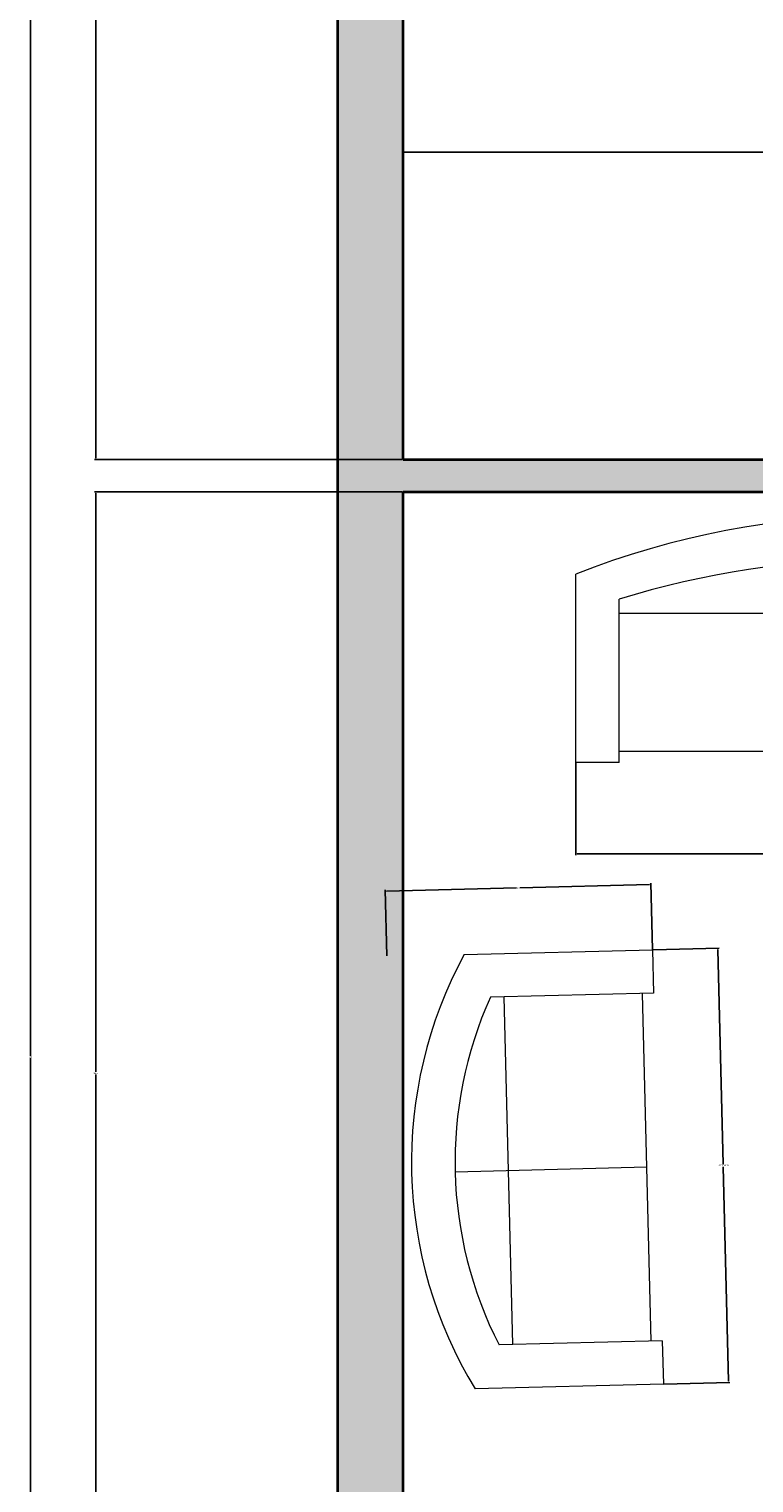
# Model space of a CAD drawing. Units: inches. Extents: x 1563 to 2428, y 777 to 1464.
# Tile 3 of 11: x 1563 to 1663, y 1063 to 1263. Entities that reach past the tile are written whole.
import ezdxf

# ---------------------------------------------------------------- set-up
doc = ezdxf.new("R2010")
doc.units = ezdxf.units.IN
for name, color, linetype, lineweight in [('A-ANNO-DIMS', 2, 'Continuous', 18), ('A-FURN', 9, 'Continuous', 18), ('A-WALL', 7, 'Continuous', 35), ('A-WALL-PATT', 8, 'Continuous', 13)]:
    doc.layers.add(name, color=color, linetype=linetype, lineweight=lineweight)
doc.styles.get("Standard").update_dxf_attribs({"font": 'arial.ttf'})
doc.dimstyles.get("Standard").update_dxf_attribs({"dimtxt": 0.18, "dimasz": 0.18, "dimexe": 0.18, "dimexo": 0.0625, "dimgap": 0.09, "dimtad": 0, "dimtih": 1, "dimtoh": 1, "dimdec": 4, "dimzin": 0, "dimdsep": 46, "dimtxsty": 'Standard', "dimcen": 0.09, "dimadec": 0, "dimazin": 0, "dimtfac": 1, "dimtdec": 4, "dimtofl": 0, "dimtmove": 0, "dimatfit": 3, "dimfxl": 1, "dimtolj": 1, "dimtzin": 0, "dimarcsym": 0})

# ---------------------------------------------------------------- blocks, each defined once
blk = doc.blocks.new('Sofa - Roundback 7 ft.')
for p, q in [((-12.00002, -32.4421), (-12.00003, -6.5971)), ((11.99997, -32.4421), (11.99998, -6.5971)), ((-36.000027, -34), (-36.000027, -11.4696)), ((35.99998, -34), (35.99998, -11.4696)), ((-35.999844, -13.3819), (35.9998, -13.3819)), ((-36.000027, -32.4421), (35.99998, -32.4421))]:
    blk.add_line(p, q)
for points in [[(-36.000027, -34), (-42.000027, -34), (-42.000027, -8)], [(41.99998, -8), (41.99998, -34), (35.99998, -34)]]:
    blk.add_lwpolyline(points)
for centre, radius, start, end in [((0, -114.25), 114.25, 68.43141, 111.5686), ((-0.00001, -127.1968), 121.1968, 72.72033, 107.2797)]:
    blk.add_arc(centre, radius, start, end)
blk = doc.blocks.new('Sofa - Roundback Loveseat 5 ft.')
for p, q in [((0, -32.44198), (0, -5.99998)), ((-24, -33.99998), (-24, -11.46958)), ((24.00004, -33.99998), (24.00004, -11.46958)), ((-23.9998, -13.38178), (23.99986, -13.38178)), ((-24, -32.44198), (24.00004, -32.44198))]:
    blk.add_line(p, q)
for points in [[(-24, -33.99998), (-30, -33.99998), (-30, -7.99998)], [(30.00004, -7.99998), (30.00004, -33.99998), (24.00004, -33.99998)]]:
    blk.add_lwpolyline(points)
for centre, radius, start, end in [((0, -60.24998), 60.24998, 60.13715, 119.8628), ((0, -61.38438), 55.38444, 64.32083, 115.6792)]:
    blk.add_arc(centre, radius, start, end)
blk = doc.blocks.new('*D24')
at = {"layer": 'A-ANNO-DIMS', "color": 0, "lineweight": -2, "transparency": 16777216}
for p, q in [((1637.93, 1162.02), (1637.93, 1149.31)), ((1721.93, 1162.02), (1721.93, 1149.31)), ((1638.11, 1149.49), (1679.34, 1149.49)), ((1721.75, 1149.49), (1680.53, 1149.49))]:
    blk.add_line(p, q, dxfattribs=at)
at = {"layer": 'A-ANNO-DIMS', "color": 0, "transparency": 16777216}
for points in [[(1638.11, 1149.52), (1638.11, 1149.46), (1637.93, 1149.49)], [(1721.75, 1149.52), (1721.75, 1149.46), (1721.93, 1149.49)]]:
    blk.add_solid(points, dxfattribs=at)
at = {"layer": 'Defpoints', "color": 0, "transparency": 16777216}
for p in [(1637.93, 1162.09), (1721.93, 1162.09), (1721.93, 1149.49)]:
    blk.add_point(p, dxfattribs=at)
at = {"layer": 'A-ANNO-DIMS', "color": 0, "transparency": 16777216, "insert": (1679.93, 1149.49), "char_height": 0.18, "attachment_point": 5}
blk.add_mtext('\\A1;SOFA 84', dxfattribs=at)
blk = doc.blocks.new('*D28')
at = {"layer": 'A-ANNO-DIMS', "color": 0, "lineweight": -2, "transparency": 16777216}
for p, q in [((1648.6, 1136.23), (1657.71, 1136.46)), ((1657.54, 1136.28), (1658.27, 1106.65)), ((1659.02, 1076.66), (1658.28, 1106.28)), ((1650.09, 1076.25), (1659.21, 1076.48))]:
    blk.add_line(p, q, dxfattribs=at)
at = {"layer": 'A-ANNO-DIMS', "color": 0, "transparency": 16777216}
for points in [[(1657.57, 1136.28), (1657.51, 1136.28), (1657.53, 1136.46)], [(1659.05, 1076.66), (1658.99, 1076.65), (1659.03, 1076.48)]]:
    blk.add_solid(points, dxfattribs=at)
at = {"layer": 'Defpoints', "color": 0, "transparency": 16777216}
for p in [(1648.53, 1136.23), (1657.53, 1136.46), (1650.03, 1076.25)]:
    blk.add_point(p, dxfattribs=at)
at = {"layer": 'A-ANNO-DIMS', "color": 0, "transparency": 16777216, "insert": (1658.28, 1106.47), "char_height": 0.18, "attachment_point": 5}
blk.add_mtext('\\A1;LOVESEAT 60', dxfattribs=at)
blk = doc.blocks.new('*D29')
at = {"layer": 'A-ANNO-DIMS', "color": 0, "lineweight": -2, "transparency": 16777216}
for p, q in [((1611.88, 1135.38), (1611.65, 1144.5)), ((1611.83, 1144.32), (1629.76, 1144.77)), ((1648.13, 1145.23), (1630.2, 1144.78)), ((1648.53, 1136.29), (1648.3, 1145.41))]:
    blk.add_line(p, q, dxfattribs=at)
at = {"layer": 'A-ANNO-DIMS', "color": 0, "transparency": 16777216}
for points in [[(1611.83, 1144.35), (1611.83, 1144.29), (1611.65, 1144.32)], [(1648.13, 1145.26), (1648.13, 1145.2), (1648.31, 1145.23)]]:
    blk.add_solid(points, dxfattribs=at)
at = {"layer": 'Defpoints', "color": 0, "transparency": 16777216}
for p in [(1611.65, 1144.32), (1648.53, 1136.23), (1611.88, 1135.32)]:
    blk.add_point(p, dxfattribs=at)
at = {"layer": 'A-ANNO-DIMS', "color": 0, "transparency": 16777216, "insert": (1629.98, 1144.77), "char_height": 0.18, "attachment_point": 5}
blk.add_mtext('\\A1;37', dxfattribs=at)
blk = doc.blocks.new('*D49')
at = {"layer": 'A-ANNO-DIMS', "color": 0, "lineweight": -2, "transparency": 16777216}
for p, q in [((1605.04, 1421.43), (1562.53, 1421.43)), ((1562.71, 1421.25), (1562.71, 1121.61)), ((1562.71, 821.61), (1562.71, 1121.25)), ((1605.04, 821.43), (1562.53, 821.43))]:
    blk.add_line(p, q, dxfattribs=at)
at = {"layer": 'A-ANNO-DIMS', "color": 0, "transparency": 16777216}
for points in [[(1562.68, 1421.25), (1562.74, 1421.25), (1562.71, 1421.43)], [(1562.68, 821.61), (1562.74, 821.61), (1562.71, 821.43)]]:
    blk.add_solid(points, dxfattribs=at)
at = {"layer": 'Defpoints', "color": 0, "transparency": 16777216}
for p in [(1562.71, 1421.43), (1605.11, 1421.43), (1605.11, 821.43)]:
    blk.add_point(p, dxfattribs=at)
at = {"layer": 'A-ANNO-DIMS', "color": 0, "transparency": 16777216, "insert": (1562.71, 1121.43), "char_height": 0.18, "attachment_point": 5}
blk.add_mtext('\\A1;600', dxfattribs=at)
blk = doc.blocks.new('*D55')
at = {"layer": 'A-ANNO-DIMS', "color": 0, "lineweight": -2, "transparency": 16777216}
for p, q in [((1614.04, 1335.93), (1571.53, 1335.93)), ((1571.71, 1335.75), (1571.71, 1270.11)), ((1571.71, 1204.11), (1571.71, 1269.75)), ((1614.04, 1203.93), (1571.53, 1203.93))]:
    blk.add_line(p, q, dxfattribs=at)
at = {"layer": 'A-ANNO-DIMS', "color": 0, "transparency": 16777216}
for points in [[(1571.68, 1335.75), (1571.74, 1335.75), (1571.71, 1335.93)], [(1571.68, 1204.11), (1571.74, 1204.11), (1571.71, 1203.93)]]:
    blk.add_solid(points, dxfattribs=at)
at = {"layer": 'Defpoints', "color": 0, "transparency": 16777216}
for p in [(1571.71, 1335.93), (1614.11, 1335.93), (1614.11, 1203.93)]:
    blk.add_point(p, dxfattribs=at)
at = {"layer": 'A-ANNO-DIMS', "color": 0, "transparency": 16777216, "insert": (1571.71, 1269.93), "char_height": 0.18, "attachment_point": 5}
blk.add_mtext('\\A1;132', dxfattribs=at)
blk = doc.blocks.new('*D56')
at = {"layer": 'A-ANNO-DIMS', "color": 0, "lineweight": -2, "transparency": 16777216}
for p, q in [((1614.11, 1203.99), (1614.11, 1246.51)), ((1614.29, 1246.33), (1673.83, 1246.33)), ((1733.93, 1246.33), (1674.39, 1246.33)), ((1734.11, 1203.99), (1734.11, 1246.51))]:
    blk.add_line(p, q, dxfattribs=at)
at = {"layer": 'A-ANNO-DIMS', "color": 0, "transparency": 16777216}
for points in [[(1614.29, 1246.36), (1614.29, 1246.3), (1614.11, 1246.33)], [(1733.93, 1246.36), (1733.93, 1246.3), (1734.11, 1246.33)]]:
    blk.add_solid(points, dxfattribs=at)
at = {"layer": 'Defpoints', "color": 0, "transparency": 16777216}
for p in [(1734.11, 1246.33), (1614.11, 1203.93), (1734.11, 1203.93)]:
    blk.add_point(p, dxfattribs=at)
at = {"layer": 'A-ANNO-DIMS', "color": 0, "transparency": 16777216, "insert": (1674.11, 1246.33), "char_height": 0.18, "attachment_point": 5}
blk.add_mtext('\\A1;120', dxfattribs=at)
blk = doc.blocks.new('*D58')
at = {"layer": 'A-ANNO-DIMS', "color": 0, "lineweight": -2, "transparency": 16777216}
for p, q in [((1614.04, 1199.43), (1571.53, 1199.43)), ((1571.71, 1199.25), (1571.71, 1119.36)), ((1571.71, 1039.11), (1571.71, 1119)), ((1614.04, 1038.93), (1571.53, 1038.93))]:
    blk.add_line(p, q, dxfattribs=at)
at = {"layer": 'A-ANNO-DIMS', "color": 0, "transparency": 16777216}
for points in [[(1571.68, 1199.25), (1571.74, 1199.25), (1571.71, 1199.43)], [(1571.68, 1039.11), (1571.74, 1039.11), (1571.71, 1038.93)]]:
    blk.add_solid(points, dxfattribs=at)
at = {"layer": 'Defpoints', "color": 0, "transparency": 16777216}
for p in [(1571.71, 1199.43), (1614.11, 1199.43), (1614.11, 1038.93)]:
    blk.add_point(p, dxfattribs=at)
at = {"layer": 'A-ANNO-DIMS', "color": 0, "transparency": 16777216, "insert": (1571.71, 1119.18), "char_height": 0.18, "attachment_point": 5}
blk.add_mtext('\\A1;160.5', dxfattribs=at)

msp = doc.modelspace()

# ---------------------------------------------------------------- hatches: boundary and pattern name
at = {"layer": 'A-WALL-PATT'}
h = msp.add_hatch(color=256, dxfattribs=at)
h.dxf.hatch_style = 1
h.paths.add_polyline_path([(1965.105, 1421.428), (1605.105, 1421.428), (1605.105, 821.428), (1965.105, 821.428)])
h.paths.add_polyline_path([(1614.105, 1199.428), (1704.105, 1199.428), (1738.605, 1199.428), (1738.605, 1251.928), (1734.105, 1251.928), (1734.105, 1203.928), (1704.105, 1203.928), (1614.105, 1203.928), (1614.105, 1335.928), (1665.105, 1335.928), (1665.105, 1340.428), (1614.105, 1340.428), (1614.105, 1412.428), (1704.105, 1412.428), (1704.105, 1340.428), (1701.105, 1340.428), (1701.105, 1335.928), (1704.105, 1335.928), (1768.605, 1335.928), (1768.605, 1340.428), (1708.605, 1340.428), (1708.605, 1412.428), (1807.605, 1412.428), (1807.605, 1340.428), (1804.605, 1340.428), (1804.605, 1335.928), (1807.605, 1335.928), (1807.605, 1275.928), (1815.105, 1275.928), (1815.105, 1280.428), (1812.105, 1280.428), (1812.105, 1412.428), (1956.105, 1412.428), (1956.105, 1280.428), (1854.105, 1280.428), (1854.105, 1275.928), (1956.105, 1275.928), (1956.105, 830.428), (1614.105, 830.428)], flags=16)
h.paths.add_polyline_path([(1917.224, 1038.928), (1917.224, 1043.846, -0.4014527), (1951.591, 1079.751), (1951.591, 1079.786), (1953.163, 1079.786), (1953.163, 1043.846), (1953.163, 1038.455), (1953.105, 1034.428), (1953.105, 1038.928), (1953.163, 1043.846), (1951.591, 1043.846), (1951.591, 1079.751, 0.4014527), (1917.224, 1043.846), (1917.224, 1038.455), (1917.224, 1034.428), (1834.605, 1034.428), (1834.605, 906.928), (1858.605, 906.928), (1858.605, 954.928), (1932.105, 954.928), (1932.105, 902.428), (1834.605, 902.428), (1834.605, 1034.428), (1914.224, 1034.428), (1914.224, 1038.928)], flags=0)
edge = h.paths.add_edge_path(flags=0)
edge.add_ellipse((1674.345, 1004.483), major_axis=(1.48, 0), ratio=0.8423039, start_angle=90, end_angle=180, ccw=False)
edge.add_line((1674.345, 1005.73), (1674.921, 1005.73))
edge.add_ellipse((2202.617, 985.642), major_axis=(528.234, 0), ratio=0.8423039, start_angle=176.34957, end_angle=177.82005, ccw=False)
edge.add_ellipse((1739.278, 760.804), major_axis=(-313.308, 0), ratio=0.8423039, start_angle=-77.87403, end_angle=-76.21947, ccw=False)
edge.add_ellipse((1739.278, 767.659), major_axis=(305.303, 0), ratio=0.8423039, start_angle=100.20954, end_angle=102.44463, ccw=False)
edge.add_ellipse((1659.357, 1231.328), major_axis=(250.96, 0), ratio=0.8423039, start_angle=-80.74343, end_angle=-77.44507)
edge.add_line((1705.625, 1023.567), (1711.685, 1026.918))
edge.add_ellipse((1711.754, 1026.21), major_axis=(0.74, 0), ratio=0.8423039, start_angle=52.06687, end_angle=90, ccw=False)
edge.add_line((1712.16, 1026.731), (1717.882, 1023.567))
edge.add_ellipse((1764.151, 1231.328), major_axis=(250.96, 0), ratio=0.8423039, start_angle=257.44507, end_angle=260.74343)
edge.add_ellipse((1684.229, 767.659), major_axis=(305.303, 0), ratio=0.8423039, start_angle=77.55537, end_angle=79.79046, ccw=False)
edge.add_ellipse((1684.229, 760.804), major_axis=(-313.308, 0), ratio=0.8423039, start_angle=256.21947, end_angle=257.87403, ccw=False)
edge.add_ellipse((1220.891, 985.642), major_axis=(-528.234, 0), ratio=0.8423039, start_angle=182.17995, end_angle=183.65043, ccw=False)
edge.add_line((1748.586, 1005.73), (1749.162, 1005.73))
edge.add_ellipse((1749.162, 1004.483), major_axis=(-1.48, 0), ratio=0.8423039, start_angle=180, end_angle=270, ccw=False)
edge.add_line((1750.642, 1004.483), (1750.642, 980.28))
edge.add_ellipse((1749.162, 980.28), major_axis=(1.48, 0), ratio=0.8423039, start_angle=270, end_angle=360, ccw=False)
edge.add_ellipse((-8843.864, 962.352), major_axis=(10593.026, 0), ratio=0.84230387, start_angle=-0.3241203, end_angle=0.0902291, ccw=False)
edge.add_ellipse((-8843.864, 962.352), major_axis=(10593.026, 0), ratio=0.84230387, start_angle=-0.3838668, end_angle=-0.3241203, ccw=False)
edge.add_ellipse((1749.162, 890.136), major_axis=(1.48, 0), ratio=0.8423039, start_angle=0, end_angle=90, ccw=False)
edge.add_line((1750.642, 890.136), (1750.642, 865.933))
edge.add_ellipse((1749.162, 865.933), major_axis=(1.48, 0), ratio=0.8423039, start_angle=270, end_angle=360, ccw=False)
edge.add_line((1749.162, 864.686), (1748.528, 864.686))
edge.add_ellipse((-8843.864, 962.352), major_axis=(10593.026, 0), ratio=0.84230387, start_angle=-0.6186432, end_angle=-0.5282715, ccw=False)
edge.add_ellipse((1747.592, 846.206), major_axis=(-2.22, 0), ratio=0.8423039, start_angle=179.37176, end_angle=248.46476, ccw=False)
edge.add_ellipse((-8844.604, 962.352), major_axis=(-10595.313, 0), ratio=0.842303864, start_angle=179.3534459, end_angle=179.3717628, ccw=False)
edge.add_ellipse((1744.512, 842.854), major_axis=(-5.246, 0), ratio=0.8423039, start_angle=90, end_angle=179.35345, ccw=False)
edge.add_line((1744.512, 838.435), (1678.995, 838.435))
edge.add_ellipse((1678.995, 842.854), major_axis=(5.246, 0), ratio=0.8423039, start_angle=180.64655, end_angle=270, ccw=False)
edge.add_ellipse((12268.111, 962.352), major_axis=(-10595.313, 0), ratio=0.84230387, start_angle=0.6282372, end_angle=0.6465541, ccw=False)
edge.add_ellipse((1675.916, 846.206), major_axis=(-2.22, 0), ratio=0.8423039, start_angle=-68.46476, end_angle=0.62824, ccw=False)
edge.add_ellipse((12267.371, 962.352), major_axis=(-10593.026, 0), ratio=0.84230387, start_angle=0.5282715, end_angle=0.6465541, ccw=False)
edge.add_line((1674.98, 864.686), (1674.345, 864.686))
edge.add_ellipse((1674.345, 865.933), major_axis=(-1.48, 0), ratio=0.8423039, start_angle=0, end_angle=90, ccw=False)
edge.add_line((1672.865, 865.933), (1672.865, 890.136))
edge.add_ellipse((1674.345, 890.136), major_axis=(1.48, 0), ratio=0.8423039, start_angle=90, end_angle=180, ccw=False)
edge.add_ellipse((12267.371, 962.352), major_axis=(-10593.026, 0), ratio=0.84230387, start_angle=0.3241203, end_angle=0.3838668, ccw=False)
edge.add_ellipse((12267.371, 962.352), major_axis=(-10593.026, 0), ratio=0.84230387, start_angle=-0.0902291, end_angle=0.3241203, ccw=False)
edge.add_ellipse((1674.345, 980.28), major_axis=(-1.48, 0), ratio=0.8423039, start_angle=0, end_angle=90, ccw=False)
edge.add_line((1672.865, 980.28), (1672.865, 1004.483))
h.paths.add_polyline_path([(1622.542, 1135.584), (1648.534, 1136.233), (1648.683, 1130.234), (1647.126, 1130.196), (1648.323, 1082.21), (1649.88, 1082.249), (1650.03, 1076.251), (1624.038, 1075.603, -0.266667)], flags=0)
edge = h.paths.add_edge_path(flags=0)
edge.add_line((1694.584, 990.705), (1700.334, 994.711))
edge.add_line((1700.334, 994.711), (1702.248, 994.711))
edge.add_line((1702.248, 994.711), (1702.248, 997.061))
edge.add_ellipse((1758.417, 997.061), major_axis=(56.169, 0), ratio=0.8423039, start_angle=150.56143, end_angle=180, ccw=False)
edge.add_ellipse((1665.091, 997.061), major_axis=(-56.169, 0), ratio=0.8423039, start_angle=180, end_angle=209.43857, ccw=False)
edge.add_line((1721.26, 997.061), (1721.26, 994.711))
edge.add_line((1721.26, 994.711), (1723.174, 994.711))
edge.add_line((1723.174, 994.711), (1728.923, 990.705))
edge.add_line((1728.923, 990.705), (1728.923, 975.895))
edge.add_ellipse((1725.091, 976.043), major_axis=(0.357, 6.34), ratio=0.6038336, start_angle=106.34259, end_angle=270.99799, ccw=False)
edge.add_line((1721.26, 975.15), (1721.26, 997.061))
edge.add_ellipse((1665.091, 997.061), major_axis=(-56.169, 0), ratio=0.8423039, start_angle=180, end_angle=209.43857)
edge.add_ellipse((1758.417, 997.061), major_axis=(56.169, 0), ratio=0.8423039, start_angle=150.56143, end_angle=180)
edge.add_line((1702.248, 997.061), (1702.248, 975.15))
edge.add_ellipse((1698.416, 976.043), major_axis=(-0.357, 6.34), ratio=0.6038336, start_angle=89.00201, end_angle=253.65741, ccw=False)
edge.add_line((1694.584, 975.895), (1694.584, 990.705))
edge = h.paths.add_edge_path(flags=0)
edge.add_line((1675.832, 952.075), (1679.883, 938.848))
edge.add_ellipse((5378.107, 931.045), major_axis=(-3698.236, 0), ratio=0.84230387, start_angle=-0.120897, end_angle=0.364076)
edge.add_line((1679.976, 907.545), (1676.149, 892.52))
edge.add_ellipse((12267.371, 962.352), major_axis=(10591.546, 0), ratio=0.84230387, start_angle=180.3241656, end_angle=180.3777642, ccw=False)
edge.add_ellipse((12267.371, 962.352), major_axis=(10591.546, 0), ratio=0.84230387, start_angle=180.0555943, end_angle=180.3241656, ccw=False)
edge = h.paths.add_edge_path(flags=0)
edge.add_ellipse((1706.366, 891.542), major_axis=(81.773, 0), ratio=0.8423039, start_angle=94.27742, end_angle=111.83495, ccw=False)
edge.add_line((1701.225, 960.283), (1722.283, 960.283))
edge.add_ellipse((1717.141, 891.542), major_axis=(-81.773, 0), ratio=0.8423039, start_angle=248.16505, end_angle=265.72258, ccw=False)
edge.add_line((1743.29, 956.803), (1741.105, 940.427))
edge.add_ellipse((1714.553, 877.238), major_axis=(79.58, 0), ratio=0.8423039, start_angle=67.20809, end_angle=85.12993)
edge.add_line((1720.25, 944.097), (1703.258, 944.097))
edge.add_ellipse((1708.954, 877.238), major_axis=(79.58, 0), ratio=0.8423039, start_angle=94.87007, end_angle=112.79191)
edge.add_line((1682.403, 940.427), (1680.218, 956.803))
h.paths.add_polyline_path([(1664.992, 1093.991), (1664.992, 1123.991), (1724.992, 1123.991), (1724.992, 1093.991)], flags=0)
h.paths.add_polyline_path([(1716.588, 1099.729), (1715.404, 1099.805), (1715.021, 1099.823), (1716.177, 1099.758)], flags=0)
h.paths.add_polyline_path([(1711.325, 1103.757), (1712.167, 1103.706), (1713.009, 1103.642), (1713.84, 1103.566), (1715.041, 1103.439), (1716.532, 1103.244), (1717.793, 1103.048), (1718.876, 1102.854), (1719.676, 1102.699), (1720.157, 1102.605), (1720.632, 1102.513), (1721.109, 1102.424), (1721.595, 1102.339), (1722.088, 1102.264), (1722.585, 1102.205), (1723.082, 1102.17), (1723.575, 1102.164), (1724.321, 1102.211), (1724.533, 1102.268), (1723.842, 1102.16), (1722.864, 1102.172), (1721.894, 1102.287), (1720.935, 1102.454), (1720.157, 1102.605), (1719.676, 1102.699), (1719.18, 1102.795), (1718.66, 1102.892), (1718.109, 1102.991), (1717.517, 1103.091), (1716.876, 1103.191), (1716.179, 1103.29), (1715.435, 1103.387), (1714.652, 1103.48), (1713.84, 1103.566), (1713.009, 1103.642), (1712.167, 1103.706), (1711.325, 1103.757), (1710.492, 1103.791), (1709.676, 1103.806), (1708.873, 1103.805), (1707.707, 1103.78), (1707.292, 1103.757), (1708.499, 1103.805), (1710.086, 1103.807)], flags=0)
h.paths.add_polyline_path([(1713.959, 1106.591), (1714.651, 1106.624), (1715.279, 1106.674), (1715.852, 1106.736), (1716.373, 1106.807), (1716.851, 1106.885), (1717.289, 1106.966), (1717.696, 1107.046), (1718.341, 1107.178), (1719.173, 1107.331), (1720.169, 1107.421), (1721.131, 1107.383), (1722.032, 1107.286), (1722.934, 1107.152), (1723.887, 1106.983), (1724.746, 1106.795), (1724.72, 1106.798), (1724.663, 1106.807), (1724.241, 1106.906), (1724.159, 1106.924), (1723.885, 1106.979), (1723.546, 1107.044), (1723.157, 1107.113), (1722.732, 1107.182), (1722.284, 1107.249), (1721.827, 1107.308), (1721.375, 1107.357), (1720.942, 1107.391), (1720.539, 1107.406), (1720.162, 1107.405), (1719.804, 1107.388), (1719.459, 1107.357), (1719.12, 1107.314), (1718.781, 1107.259), (1718.435, 1107.195), (1718.076, 1107.124), (1717.402, 1106.986), (1716.59, 1106.837), (1715.56, 1106.696), (1714.317, 1106.598)], flags=0)
h.paths.add_polyline_path([(1708.692, 1110.124), (1709.455, 1110.13), (1710.147, 1110.149), (1710.772, 1110.18), (1711.334, 1110.224), (1711.836, 1110.28), (1712.283, 1110.349), (1712.678, 1110.43), (1713.026, 1110.524), (1713.33, 1110.63), (1713.596, 1110.746), (1713.832, 1110.87), (1714.042, 1110.999), (1714.234, 1111.131), (1714.413, 1111.264), (1714.586, 1111.396), (1715.065, 1111.75), (1715.879, 1112.11), (1716.842, 1112.224), (1717.903, 1112.165), (1719.048, 1111.965), (1719.867, 1111.736), (1720.686, 1111.487), (1721.596, 1111.22), (1721.917, 1111.136), (1721.028, 1111.383), (1720.222, 1111.628), (1719.815, 1111.75), (1719.434, 1111.857), (1719.054, 1111.951), (1718.672, 1112.031), (1718.292, 1112.097), (1717.918, 1112.149), (1717.554, 1112.185), (1717.204, 1112.204), (1716.871, 1112.206), (1716.559, 1112.191), (1716.271, 1112.156), (1716.006, 1112.105), (1715.761, 1112.038), (1715.534, 1111.957), (1715.323, 1111.864), (1715.125, 1111.759), (1714.937, 1111.645), (1714.759, 1111.524), (1714.586, 1111.396), (1714.413, 1111.264), (1714.003, 1110.96), (1713.331, 1110.606), (1712.501, 1110.382), (1711.61, 1110.245), (1710.489, 1110.158), (1709.111, 1110.121)], flags=0)
h.paths.add_polyline_path([(1707.127, 1113.075), (1707.639, 1113.025), (1708.092, 1112.991), (1708.49, 1112.975), (1708.836, 1112.977), (1709.135, 1112.996), (1709.392, 1113.032), (1709.612, 1113.084), (1709.798, 1113.15), (1709.957, 1113.23), (1710.092, 1113.324), (1710.208, 1113.431), (1710.304, 1113.554), (1710.379, 1113.698), (1710.434, 1113.866), (1710.467, 1114.062), (1710.477, 1114.289), (1710.463, 1114.553), (1710.426, 1114.857), (1710.364, 1115.202), (1710.282, 1115.58), (1710.184, 1115.98), (1710.076, 1116.391), (1709.961, 1116.801), (1709.844, 1117.201), (1709.731, 1117.579), (1709.626, 1117.924), (1709.532, 1118.228), (1709.454, 1118.493), (1709.392, 1118.723), (1709.351, 1118.924), (1709.293, 1119.435), (1709.831, 1119.942), (1710.705, 1120.121), (1711.507, 1119.898), (1712.224, 1119.567), (1713.189, 1119.016), (1713.529, 1118.804), (1712.958, 1119.148), (1712.468, 1119.428), (1712.046, 1119.649), (1711.683, 1119.817), (1711.366, 1119.937), (1711.084, 1120.016), (1710.826, 1120.057), (1710.582, 1120.067), (1710.354, 1120.049), (1710.142, 1120.006), (1709.951, 1119.941), (1709.781, 1119.857), (1709.635, 1119.757), (1709.516, 1119.645), (1709.426, 1119.524), (1709.366, 1119.395), (1709.335, 1119.255), (1709.331, 1119.1), (1709.351, 1118.924), (1709.392, 1118.723), (1709.454, 1118.493), (1709.52, 1118.268), (1709.799, 1117.356), (1710.028, 1116.57), (1710.245, 1115.749), (1710.45, 1114.804), (1710.477, 1114.289), (1710.448, 1113.654), (1709.908, 1113.153), (1709.165, 1112.979), (1708.318, 1112.974), (1707.448, 1113.039)], flags=0)
h.paths.add_polyline_path([(1700.892, 1119.857), (1701.604, 1119.819), (1702.196, 1119.805), (1702.683, 1119.813), (1703.076, 1119.841), (1703.387, 1119.887), (1703.63, 1119.951), (1703.816, 1120.03), (1703.959, 1120.124), (1704.069, 1120.23), (1704.15, 1120.346), (1704.204, 1120.47), (1704.234, 1120.599), (1704.242, 1120.731), (1704.231, 1120.864), (1704.202, 1120.996), (1704.159, 1121.124), (1704.103, 1121.246), (1704.039, 1121.362), (1703.97, 1121.474), (1703.901, 1121.582), (1703.834, 1121.687), (1703.775, 1121.79), (1703.564, 1122.226), (1704.048, 1122.698), (1704.756, 1122.769), (1705.49, 1122.723), (1706.24, 1122.641), (1706.547, 1122.601), (1706.092, 1122.657), (1705.695, 1122.701), (1705.348, 1122.732), (1705.049, 1122.751), (1704.792, 1122.757), (1704.573, 1122.751), (1704.386, 1122.732), (1704.227, 1122.701), (1704.092, 1122.657), (1703.977, 1122.601), (1703.88, 1122.534), (1703.802, 1122.458), (1703.742, 1122.374), (1703.702, 1122.284), (1703.68, 1122.188), (1703.677, 1122.09), (1703.692, 1121.991), (1703.726, 1121.89), (1703.769, 1121.802), (1704.039, 1121.362), (1704.301, 1120.887), (1704.133, 1120.165), (1703.43, 1119.866), (1702.481, 1119.798), (1701.306, 1119.827)], flags=0)
edge = h.paths.add_edge_path(flags=0)
edge.add_ellipse((1711.754, 1009.752), major_axis=(-147.018, 0), ratio=0.8423039, start_angle=76.40187, end_angle=103.59813)
edge.add_line((1741.105, 888.411), (1741.105, 869.587))
edge.add_ellipse((1711.754, 990.928), major_axis=(-147.018, 0), ratio=0.8423039, start_angle=76.40187, end_angle=103.59813, ccw=False)
edge.add_line((1682.403, 869.587), (1682.403, 888.411))
edge = h.paths.add_edge_path(flags=0)
edge.add_ellipse((-8843.864, 962.352), major_axis=(-10591.546, 0), ratio=0.84230387, start_angle=179.6758344, end_angle=179.9444057, ccw=False)
edge.add_ellipse((-8843.864, 962.352), major_axis=(-10591.546, 0), ratio=0.84230387, start_angle=179.6222358, end_angle=179.6758344, ccw=False)
edge.add_line((1747.358, 892.52), (1743.531, 907.545))
edge.add_ellipse((-1954.6, 931.045), major_axis=(3698.236, 0), ratio=0.84230387, start_angle=-0.364076, end_angle=0.120897)
edge.add_line((1743.625, 938.848), (1747.676, 952.075))
h.paths.add_polyline_path([(1637.931, 1162.087), (1637.931, 1188.087, -0.1904762), (1721.931, 1188.087), (1721.931, 1162.087), (1715.931, 1162.087), (1715.931, 1163.644), (1643.931, 1163.644), (1643.931, 1162.087)], flags=0)
h.paths.add_polyline_path([(1667.931, 1189.491, -0.0496282), (1691.931, 1189.491), (1691.931, 1182.705), (1667.931, 1182.705)], flags=0)
edge = h.paths.add_edge_path(flags=0)
edge.add_ellipse((1685.362, 859.825), major_axis=(-2.96, 0), ratio=0.8423039, start_angle=-90, end_angle=0, ccw=False)
edge.add_line((1685.362, 862.318), (1738.145, 862.318))
edge.add_ellipse((1738.145, 859.825), major_axis=(2.96, 0), ratio=0.8423039, start_angle=0, end_angle=90, ccw=False)
edge.add_line((1741.105, 859.825), (1741.105, 840.361))
edge.add_line((1741.105, 840.361), (1682.403, 840.361))
edge.add_line((1682.403, 840.361), (1682.403, 859.825))
h.paths.add_polyline_path([(1777.486, 1164.853), (1777.486, 1180.853), (1778.486, 1181.01), (1778.486, 1164.697)], flags=0)
h.paths.add_polyline_path([(1786.986, 1154.853), (1786.986, 1163.369), (1778.986, 1164.619), (1778.986, 1181.088), (1786.986, 1182.338), (1786.986, 1190.853), (1799.502, 1190.853), (1800.752, 1198.853), (1817.221, 1198.853), (1818.471, 1190.853), (1827.502, 1190.853), (1828.752, 1198.853), (1845.221, 1198.853), (1846.471, 1190.853), (1858.986, 1190.853), (1858.986, 1182.338), (1866.986, 1181.088), (1866.986, 1164.619), (1858.986, 1163.369), (1858.986, 1154.853), (1846.471, 1154.853), (1845.221, 1146.853), (1828.752, 1146.853), (1827.502, 1154.853), (1818.471, 1154.853), (1817.221, 1146.853), (1800.752, 1146.853), (1799.502, 1154.853)], flags=0)
h.paths.add_polyline_path([(1800.986, 1145.353), (1800.83, 1146.353), (1817.143, 1146.353), (1816.986, 1145.353)], flags=0)
h.paths.add_polyline_path([(1851.408, 1167.858), (1852.086, 1167.738), (1852.744, 1167.621), (1853.388, 1167.506), (1854.028, 1167.395), (1854.67, 1167.289), (1855.313, 1167.195), (1855.952, 1167.122), (1856.585, 1167.077), (1857.209, 1167.07), (1858.147, 1167.128), (1858.413, 1167.2), (1857.547, 1167.066), (1856.312, 1167.08), (1855.07, 1167.223), (1854.028, 1167.395), (1853.388, 1167.506), (1852.744, 1167.621), (1852.086, 1167.738), (1851.408, 1167.858), (1850.288, 1168.052), (1849.956, 1168.104), (1850.701, 1167.98)], flags=0)
h.paths.add_polyline_path([(1845.435, 1172.646), (1846.222, 1172.707), (1846.941, 1172.785), (1847.601, 1172.874), (1848.21, 1172.971), (1848.777, 1173.072), (1849.311, 1173.173), (1850.14, 1173.331), (1851.063, 1173.483), (1852.014, 1173.591), (1853.012, 1173.633), (1854.075, 1173.594), (1855.251, 1173.473), (1856.4, 1173.306), (1857.391, 1173.132), (1857.945, 1173.02), (1858.196, 1172.965), (1858.595, 1172.871), (1858.575, 1172.874), (1858.49, 1172.894), (1858.371, 1172.924), (1858.196, 1172.965), (1857.945, 1173.02), (1857.602, 1173.089), (1857.177, 1173.17), (1856.687, 1173.256), (1856.148, 1173.343), (1855.575, 1173.426), (1854.986, 1173.5), (1854.395, 1173.561), (1853.82, 1173.603), (1853.272, 1173.623), (1852.749, 1173.622), (1852.247, 1173.6), (1851.757, 1173.562), (1851.276, 1173.507), (1850.796, 1173.439), (1850.313, 1173.359), (1849.82, 1173.27), (1849.311, 1173.173), (1848.421, 1173.005), (1847.25, 1172.818), (1845.826, 1172.665)], flags=0)
h.paths.add_polyline_path([(1840.587, 1177.09), (1841.289, 1177.145), (1841.916, 1177.215), (1842.475, 1177.301), (1842.969, 1177.403), (1843.403, 1177.52), (1843.783, 1177.652), (1844.117, 1177.797), (1844.411, 1177.952), (1844.674, 1178.114), (1844.914, 1178.279), (1845.138, 1178.446), (1845.644, 1178.831), (1846.285, 1179.221), (1847.125, 1179.521), (1847.998, 1179.624), (1848.834, 1179.619), (1849.768, 1179.529), (1850.775, 1179.363), (1851.78, 1179.14), (1852.111, 1179.053), (1851.57, 1179.187), (1851.043, 1179.304), (1850.527, 1179.404), (1850.024, 1179.487), (1849.539, 1179.551), (1849.072, 1179.596), (1848.628, 1179.62), (1848.21, 1179.623), (1847.82, 1179.603), (1847.46, 1179.561), (1847.128, 1179.497), (1846.822, 1179.413), (1846.539, 1179.312), (1846.274, 1179.195), (1846.027, 1179.064), (1845.793, 1178.922), (1845.57, 1178.77), (1845.354, 1178.61), (1844.817, 1178.201), (1844.106, 1177.764), (1843.208, 1177.452), (1842.225, 1177.25), (1840.973, 1177.11)], flags=0)
h.paths.add_polyline_path([(1836.67, 1180.646), (1837.236, 1180.603), (1837.734, 1180.584), (1838.166, 1180.586), (1838.54, 1180.611), (1838.861, 1180.655), (1839.136, 1180.72), (1839.369, 1180.803), (1839.568, 1180.903), (1839.736, 1181.02), (1839.881, 1181.152), (1840.001, 1181.299), (1840.095, 1181.456), (1840.164, 1181.624), (1840.204, 1181.8), (1840.217, 1181.981), (1840.2, 1182.166), (1840.153, 1182.353), (1840.076, 1182.541), (1839.973, 1182.728), (1839.851, 1182.916), (1839.716, 1183.103), (1839.572, 1183.291), (1839.427, 1183.478), (1839.033, 1184), (1838.862, 1184.411), (1838.695, 1184.99), (1839.2, 1185.669), (1840.06, 1185.961), (1840.793, 1185.931), (1841.454, 1185.77), (1842.179, 1185.536), (1842.706, 1185.363), (1843.713, 1185.044), (1844.033, 1184.956), (1843.102, 1185.234), (1842.179, 1185.536), (1841.725, 1185.682), (1841.328, 1185.801), (1840.976, 1185.886), (1840.653, 1185.937), (1840.349, 1185.949), (1840.063, 1185.926), (1839.799, 1185.872), (1839.559, 1185.791), (1839.347, 1185.686), (1839.165, 1185.562), (1839.016, 1185.422), (1838.903, 1185.27), (1838.828, 1185.11), (1838.79, 1184.943), (1838.784, 1184.77), (1838.809, 1184.593), (1838.862, 1184.411), (1838.938, 1184.227), (1839.036, 1184.041), (1839.153, 1183.853), (1839.285, 1183.666), (1839.427, 1183.478), (1839.572, 1183.291), (1839.716, 1183.103), (1839.851, 1182.916), (1840.178, 1182.415), (1840.251, 1181.604), (1839.686, 1180.915), (1838.893, 1180.633), (1837.976, 1180.574), (1837.01, 1180.612)], flags=0)
h.paths.add_polyline_path([(1829.867, 1185.622), (1830.475, 1185.631), (1830.966, 1185.666), (1831.355, 1185.724), (1831.658, 1185.804), (1831.891, 1185.903), (1832.07, 1186.02), (1832.207, 1186.152), (1832.308, 1186.297), (1832.376, 1186.452), (1832.414, 1186.614), (1832.424, 1186.779), (1832.41, 1186.946), (1832.374, 1187.11), (1832.32, 1187.27), (1832.25, 1187.422), (1832.17, 1187.568), (1832.084, 1187.708), (1831.997, 1187.843), (1831.914, 1187.974), (1831.839, 1188.102), (1831.614, 1188.57), (1832.036, 1189.169), (1832.801, 1189.319), (1833.589, 1189.3), (1834.44, 1189.223), (1834.736, 1189.187), (1834.239, 1189.241), (1833.807, 1189.28), (1833.433, 1189.304), (1833.111, 1189.312), (1832.837, 1189.304), (1832.604, 1189.28), (1832.405, 1189.241), (1832.236, 1189.187), (1832.092, 1189.117), (1831.971, 1189.033), (1831.873, 1188.938), (1831.799, 1188.832), (1831.748, 1188.719), (1831.721, 1188.601), (1831.717, 1188.478), (1831.736, 1188.353), (1831.779, 1188.228), (1831.839, 1188.102), (1831.914, 1187.974), (1831.997, 1187.843), (1832.084, 1187.708), (1832.387, 1187.216), (1832.456, 1186.393), (1831.916, 1185.871), (1831.195, 1185.682), (1830.221, 1185.613)], flags=0)
h.paths.add_polyline_path([(1828.986, 1145.353), (1828.83, 1146.353), (1845.143, 1146.353), (1844.986, 1145.353)], flags=0)
h.paths.add_polyline_path([(1800.986, 1200.353), (1816.986, 1200.353), (1817.143, 1199.353), (1800.83, 1199.353)], flags=0)
h.paths.add_polyline_path([(1828.986, 1200.353), (1844.986, 1200.353), (1845.143, 1199.353), (1828.83, 1199.353)], flags=0)
h.paths.add_polyline_path([(1867.486, 1181.01), (1868.486, 1180.853), (1868.486, 1164.853), (1867.486, 1164.697)], flags=0)
h.paths.add_polyline_path([(1901.055, 1112.089), (1901.055, 1241.889), (1954.299, 1241.889), (1954.299, 1112.089)], flags=0)
h.paths.add_polyline_path([(1908.544, 1229.408), (1931.009, 1229.408), (1937.23, 1216.927), (1931.009, 1216.927), (1931.009, 1129.562), (1908.544, 1129.562)], flags=0)
h.paths.add_polyline_path([(1699.472, 1381.538), (1701.045, 1381.538), (1701.045, 1345.599), (1699.472, 1345.599)], flags=0)
h.paths.add_polyline_path([(1851.045, 1285.819), (1851.045, 1280.428), (1851.105, 1275.928), (1851.105, 1280.428)], flags=0)
h.paths.add_polyline_path([(1815.105, 1285.819), (1815.105, 1321.758), (1816.678, 1321.758), (1816.678, 1285.819)], flags=0)
h.paths.add_polyline_path([(1745.154, 1343.707, -0.1044693), (1742.568, 1347.148, -0.1176343), (1741.799, 1350.905, -0.1176343), (1742.808, 1354.603, -0.1044693), (1745.61, 1357.871, -0.0900158), (1749.544, 1359.891, -0.0819199), (1754.355, 1360.526, -0.0819199), (1759.115, 1359.583, -0.0900158), (1762.911, 1357.314, -0.1044693), (1765.497, 1353.872, -0.1176343), (1766.266, 1350.116, -0.1176343), (1765.257, 1346.417, -0.1044693), (1762.455, 1343.149, -0.0900158), (1758.521, 1341.13, -0.0819199), (1753.71, 1340.495, -0.0819199), (1748.95, 1341.438, -0.0900158)], flags=0)
h.paths.add_polyline_path([(1745.961, 1344.152, -0.1046782), (1743.517, 1347.257, -0.1186217), (1742.746, 1350.669, -0.1186217), (1743.612, 1354.059, -0.1046782), (1746.143, 1357.094, -0.0895621), (1749.732, 1359.002, -0.0811847), (1754.161, 1359.662, -0.0811847), (1758.57, 1358.877, -0.0895621), (1762.104, 1356.869, -0.1046782), (1764.548, 1353.764, -0.1186217), (1765.319, 1350.351, -0.1186217), (1764.453, 1346.962, -0.1046782), (1761.922, 1343.927, -0.0895621), (1758.333, 1342.019, -0.0811847), (1753.904, 1341.359, -0.0811847), (1749.495, 1342.143, -0.0895621)], flags=0)
h.paths.add_polyline_path([(1748.738, 1346.3, -0.1046075), (1747.125, 1348.343, -0.1182826), (1746.612, 1350.593, -0.1182826), (1747.176, 1352.832, -0.1046075), (1748.833, 1354.838, -0.089718), (1751.19, 1356.103, -0.0814361), (1754.1, 1356.547, -0.0814361), (1756.999, 1356.038, -0.089718), (1759.327, 1354.72, -0.1046075), (1760.94, 1352.678, -0.1182826), (1761.453, 1350.427, -0.1182826), (1760.889, 1348.189, -0.1046075), (1759.232, 1346.183, -0.089718), (1756.875, 1344.917, -0.0814361), (1753.965, 1344.474, -0.0814361), (1751.066, 1344.982, -0.089718)], flags=0)
h.paths.add_polyline_path([(1802.972, 1381.538), (1804.545, 1381.538), (1804.545, 1345.599), (1802.972, 1345.599)], flags=0)
h.paths.add_polyline_path([(1752.533, 1350.51, -1), (1755.533, 1350.51, -1)], flags=0)
h.paths.add_polyline_path([(1753.033, 1350.51, -1), (1755.033, 1350.51, -1)], flags=0)
h.paths.add_polyline_path([(1869.759, 1336.236), (1869.759, 1396.236), (1949.759, 1396.236), (1949.759, 1336.236)], flags=0)
h.paths.add_polyline_path([(1920.159, 1336.236), (1920.159, 1351.436), (1935.359, 1351.436), (1935.359, 1388.236), (1948.559, 1388.236), (1948.559, 1367.436), (1935.359, 1367.436), (1935.359, 1365.036), (1948.559, 1365.036), (1948.559, 1344.236), (1933.359, 1344.236), (1933.359, 1349.436)], flags=0)
h.paths.add_polyline_path([(1938.156, 1328.719, -1), (1952.156, 1328.719, -1)], flags=0)
h.paths.add_polyline_path([(1942.156, 1328.719), (1945.156, 1331.719), (1948.156, 1328.719), (1945.156, 1325.719)], flags=0)
h.paths.add_polyline_path([(1944.156, 1328.719, -1), (1946.156, 1328.719, -1)], flags=0)
h.paths.add_polyline_path([(1914.224, 1038.928), (1614.105, 1038.928), (1614.105, 1034.428), (1830.105, 1034.428), (1830.105, 830.428), (1834.605, 830.428), (1834.605, 1034.428), (1914.224, 1034.428)], flags=0)
h.paths.add_polyline_path([(1956.105, 902.428), (1834.605, 902.428), (1834.605, 830.428), (1956.105, 830.428)], flags=0)

# ---------------------------------------------------------------- linework, layer by layer
at = {"layer": 'A-WALL'}
for p, q in [((1614.105, 1203.928), (1614.105, 1335.928)), ((1614.105, 830.428), (1614.105, 1199.428))]:
    msp.add_line(p, q, dxfattribs=at)
msp.add_lwpolyline([(1605.105, 1421.428), (1965.105, 1421.428), (1965.105, 821.428), (1605.105, 821.428)], close=True, dxfattribs=at)
for points in [[(1614.105, 1203.928), (1704.105, 1203.928), (1734.105, 1203.928)], [(1614.105, 1199.428), (1704.105, 1199.428), (1738.605, 1199.428)]]:
    msp.add_lwpolyline(points, dxfattribs=at)

# ---------------------------------------------------------------- block references
at = {"layer": 'A-FURN'}
msp.add_blockref('Sofa - Roundback 7 ft.', (1679.931, 1196.087), dxfattribs=at)
at = {"layer": 'A-FURN', "rotation": 91.42884202491504}
msp.add_blockref('Sofa - Roundback Loveseat 5 ft.', (1615.292, 1105.394), dxfattribs=at)

# ---------------------------------------------------------------- dimensions: what is measured, and where the dimension line sits
at = {"layer": 'A-ANNO-DIMS'}
for base, p1, p2, angle, override, picture, middle in [((1562.705, 1421.428), (1605.105, 821.428), (1605.105, 1421.428), 90, {"dimdec": 0, "dimlfac": 1, "dimrnd": 0, "dimzin": 0, "dimdsep": 46, "dimlunit": 2}, '*D49', (1562.705, 1121.428)), ((1571.705, 1335.928), (1614.105, 1203.928), (1614.105, 1335.928), 90, {"dimdec": 0, "dimlfac": 1, "dimrnd": 0, "dimzin": 0, "dimdsep": 46, "dimlunit": 2}, '*D55', (1571.705, 1269.928)), ((1734.105, 1246.328), (1614.105, 1203.928), (1734.105, 1203.928), 0, {"dimdec": 0, "dimlfac": 1, "dimrnd": 0, "dimzin": 0, "dimdsep": 46, "dimlunit": 2}, '*D56', (1674.105, 1246.328)), ((1571.705, 1199.428), (1614.105, 1038.928), (1614.105, 1199.428), 90, {"dimdec": 1, "dimlfac": 1, "dimrnd": 0, "dimzin": 0, "dimdsep": 46, "dimlunit": 2}, '*D58', (1571.705, 1119.178)), ((1611.654, 1144.315), (1648.534, 1136.233), (1611.878, 1135.318), 181.42884, {"dimdec": 0, "dimlfac": 1, "dimrnd": 0, "dimzin": 0, "dimdsep": 46, "dimlunit": 2}, '*D29', (1629.982, 1144.773))]:
    dim = msp.add_linear_dim(base=base, p1=p1, p2=p2, angle=angle, dimstyle='Standard', override=override, dxfattribs=at)
    dim.commit()
    dim.dimension.update_dxf_attribs({"geometry": picture, "text_midpoint": middle})
dim = msp.add_linear_dim(base=(1721.931, 1149.487), p1=(1637.931, 1162.087), p2=(1721.931, 1162.087), text='SOFA <>', dimstyle='Standard', override={"dimdec": 0, "dimlfac": 1, "dimrnd": 0, "dimzin": 0, "dimdsep": 46, "dimlunit": 2}, dxfattribs=at)
dim.commit()
dim.dimension.update_dxf_attribs({"geometry": '*D24', "text_midpoint": (1679.931, 1149.487)})
dim = msp.add_linear_dim(base=(1657.531, 1136.457), p1=(1650.03, 1076.251), p2=(1648.534, 1136.233), angle=91.42884, text='LOVESEAT <>', dimstyle='Standard', override={"dimdec": 0, "dimlfac": 1, "dimrnd": 0, "dimzin": 0, "dimdsep": 46, "dimlunit": 2}, dxfattribs=at)
dim.commit()
dim.dimension.update_dxf_attribs({"geometry": '*D28', "text_midpoint": (1658.279, 1106.466)})

doc.saveas('drawing.dxf')
